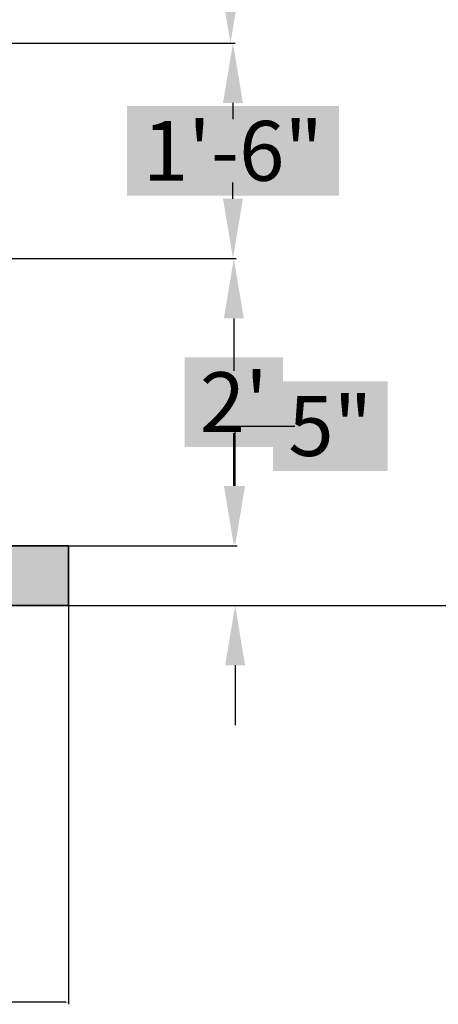
# Model space of a CAD drawing. Units: inches. Extents: x -301 to 715, y -607 to 364.
# Tile 32 of 141: x 159 to 194, y -574 to -492. Entities that reach past the tile are written whole.
import ezdxf

# ---------------------------------------------------------------- set-up
doc = ezdxf.new("R2010")
doc.units = ezdxf.units.IN
doc.header["$MEASUREMENT"] = 0
for name, color, linetype, lineweight in [('A-ANNO-DIMS', 2, 'Continuous', 18), ('A-SECT-PATT', 8, 'Continuous', 13), ('S-FNDN', 2, 'Continuous', 35)]:
    doc.layers.add(name, color=color, linetype=linetype, lineweight=lineweight)
doc.styles.get("Standard").update_dxf_attribs({"font": 'arial.ttf'})
doc.dimstyles.get("Standard").update_dxf_attribs({"dimtxt": 0.18, "dimasz": 0.18, "dimexe": 0.18, "dimexo": 0.0625, "dimgap": 0.09, "dimtad": 0, "dimtih": 1, "dimtoh": 1, "dimdec": 1, "dimzin": 0, "dimdsep": 46, "dimlunit": 4, "dimtxsty": 'Standard', "dimcen": 0.09, "dimclrd": 3, "dimclre": 4, "dimclrt": 6, "dimadec": 0, "dimazin": 0, "dimtfac": 1, "dimtdec": 1, "dimtofl": 0, "dimtmove": 0, "dimatfit": 3, "dimfxl": 1, "dimtfill": 2, "dimtfillclr": 51, "dimtolj": 1, "dimtzin": 0, "dimarcsym": 0})

# ---------------------------------------------------------------- blocks, each defined once
blk = doc.blocks.new('*D77')
at = {"layer": 'A-ANNO-DIMS', "color": 0, "lineweight": -2, "transparency": 16777216}
for p, q in [((177.201, -530.477), (177.201, -525.477)), ((177.201, -525.477), (182.201, -525.477)), ((163.318, -535.477), (177.381, -535.477)), ((163.318, -540.477), (177.381, -540.477)), ((177.201, -545.477), (177.201, -550.477))]:
    blk.add_line(p, q, dxfattribs=at)
at = {"layer": 'A-ANNO-DIMS', "color": 0, "transparency": 16777216}
for points in [[(176.368, -530.477), (178.035, -530.477), (177.201, -535.477)], [(176.368, -545.477), (178.035, -545.477), (177.201, -540.477)]]:
    blk.add_solid(points, dxfattribs=at)
at = {"layer": 'Defpoints', "color": 0, "transparency": 16777216}
for p in [(163.255, -535.477), (177.201, -535.477), (163.255, -540.477)]:
    blk.add_point(p, dxfattribs=at)
at = {"layer": 'A-ANNO-DIMS', "color": 0, "transparency": 16777216, "insert": (185.165, -525.477), "char_height": 5, "attachment_point": 5, "bg_fill": 1, "box_fill_scale": 1.25, "bg_fill_color": 51, "bg_fill_transparency": 0}
blk.add_mtext('\\A1;5"', dxfattribs=at)
blk = doc.blocks.new('*D78')
at = {"layer": 'A-ANNO-DIMS', "color": 0, "lineweight": -2, "transparency": 16777216}
for p, q in [((158.318, -511.477), (177.276, -511.477)), ((177.096, -516.477), (177.096, -520.877)), ((177.096, -530.477), (177.096, -526.078)), ((158.318, -535.477), (177.276, -535.477))]:
    blk.add_line(p, q, dxfattribs=at)
at = {"layer": 'A-ANNO-DIMS', "color": 0, "transparency": 16777216}
for points in [[(176.262, -516.477), (177.929, -516.477), (177.096, -511.477)], [(176.262, -530.477), (177.929, -530.477), (177.096, -535.477)]]:
    blk.add_solid(points, dxfattribs=at)
at = {"layer": 'Defpoints', "color": 0, "transparency": 16777216}
for p in [(158.255, -511.477), (177.096, -511.477), (158.255, -535.477)]:
    blk.add_point(p, dxfattribs=at)
at = {"layer": 'A-ANNO-DIMS', "color": 0, "transparency": 16777216, "insert": (177.096, -523.477), "char_height": 5, "attachment_point": 5, "bg_fill": 1, "box_fill_scale": 1.25, "bg_fill_color": 51, "bg_fill_transparency": 0}
blk.add_mtext("\\A1;2'", dxfattribs=at)
blk = doc.blocks.new('*D79')
at = {"layer": 'A-ANNO-DIMS', "color": 0, "lineweight": -2, "transparency": 16777216}
for p, q in [((153.318, -493.477), (177.201, -493.477)), ((177.021, -498.477), (177.021, -499.835)), ((177.021, -506.477), (177.021, -505.12)), ((153.318, -511.477), (177.201, -511.477))]:
    blk.add_line(p, q, dxfattribs=at)
at = {"layer": 'A-ANNO-DIMS', "color": 0, "transparency": 16777216}
for points in [[(176.188, -498.477), (177.854, -498.477), (177.021, -493.477)], [(176.188, -506.477), (177.854, -506.477), (177.021, -511.477)]]:
    blk.add_solid(points, dxfattribs=at)
at = {"layer": 'Defpoints', "color": 0, "transparency": 16777216}
for p in [(153.255, -493.477), (177.021, -493.477), (153.255, -511.477)]:
    blk.add_point(p, dxfattribs=at)
at = {"layer": 'A-ANNO-DIMS', "color": 0, "transparency": 16777216, "insert": (177.021, -502.477), "char_height": 5, "attachment_point": 5, "bg_fill": 1, "box_fill_scale": 1.25, "bg_fill_color": 51, "bg_fill_transparency": 0}
blk.add_mtext('\\A1;1\'-6"', dxfattribs=at)
blk = doc.blocks.new('*D80')
at = {"layer": 'A-ANNO-DIMS', "color": 0, "lineweight": -2, "transparency": 16777216}
for p, q in [((176.814, -481.477), (176.814, -476.477)), ((176.814, -476.477), (181.814, -476.477)), ((153.318, -481.477), (176.994, -481.477)), ((176.814, -488.477), (176.814, -486.477)), ((153.318, -493.477), (176.994, -493.477))]:
    blk.add_line(p, q, dxfattribs=at)
at = {"layer": 'A-ANNO-DIMS', "color": 0, "transparency": 16777216}
for points in [[(175.981, -486.477), (177.648, -486.477), (176.814, -481.477)], [(175.981, -488.477), (177.648, -488.477), (176.814, -493.477)]]:
    blk.add_solid(points, dxfattribs=at)
at = {"layer": 'Defpoints', "color": 0, "transparency": 16777216}
for p in [(153.255, -481.477), (176.814, -481.477), (153.255, -493.477)]:
    blk.add_point(p, dxfattribs=at)
at = {"layer": 'A-ANNO-DIMS', "color": 0, "transparency": 16777216, "insert": (183.969, -476.477), "char_height": 5, "attachment_point": 5, "bg_fill": 1, "box_fill_scale": 1.25, "bg_fill_color": 51, "bg_fill_transparency": 0}
blk.add_mtext("\\A1;1'", dxfattribs=at)
blk = doc.blocks.new('*D176')
at = {"layer": 'A-ANNO-DIMS', "color": 4, "lineweight": -2, "transparency": 16777216}
for p, q in [((148.28, -324.477), (215.605, -324.477)), ((-15.22, -540.477), (215.605, -540.477))]:
    blk.add_line(p, q, dxfattribs=at)
at = {"layer": 'A-ANNO-DIMS', "color": 3, "lineweight": -2, "transparency": 16777216}
for p, q in [((215.425, -324.657), (215.425, -432.296)), ((215.425, -540.297), (215.425, -432.659))]:
    blk.add_line(p, q, dxfattribs=at)
at = {"layer": 'A-ANNO-DIMS', "color": 3, "transparency": 16777216}
for points in [[(215.395, -324.657), (215.455, -324.657), (215.425, -324.477)], [(215.395, -540.297), (215.455, -540.297), (215.425, -540.477)]]:
    blk.add_solid(points, dxfattribs=at)
at = {"layer": 'Defpoints', "color": 0, "transparency": 16777216}
for p in [(148.218, -324.477), (-15.282, -540.477), (215.425, -540.477)]:
    blk.add_point(p, dxfattribs=at)
at = {"layer": 'A-ANNO-DIMS', "color": 6, "transparency": 16777216, "insert": (215.425, -432.477), "char_height": 0.18, "attachment_point": 5, "bg_fill": 1, "box_fill_scale": 1.25, "bg_fill_color": 51, "bg_fill_transparency": 0}
blk.add_mtext('\\A1;18\'-0"', dxfattribs=at)
blk = doc.blocks.new('*D182')
at = {"layer": 'A-ANNO-DIMS', "color": 4, "lineweight": -2, "transparency": 16777216}
for p, q in [((114.255, -540.54), (114.255, -573.809)), ((163.255, -540.54), (163.255, -573.809))]:
    blk.add_line(p, q, dxfattribs=at)
at = {"layer": 'A-ANNO-DIMS', "color": 3, "lineweight": -2, "transparency": 16777216}
for p, q in [((114.435, -573.629), (138.422, -573.629)), ((163.075, -573.629), (139.088, -573.629))]:
    blk.add_line(p, q, dxfattribs=at)
at = {"layer": 'A-ANNO-DIMS', "color": 3, "transparency": 16777216}
for points in [[(114.435, -573.599), (114.435, -573.659), (114.255, -573.629)], [(163.075, -573.599), (163.075, -573.659), (163.255, -573.629)]]:
    blk.add_solid(points, dxfattribs=at)
at = {"layer": 'Defpoints', "color": 0, "transparency": 16777216}
for p in [(114.255, -540.477), (163.255, -540.477), (163.255, -573.629)]:
    blk.add_point(p, dxfattribs=at)
at = {"layer": 'A-ANNO-DIMS', "color": 6, "transparency": 16777216, "insert": (138.755, -573.629), "char_height": 0.18, "attachment_point": 5, "bg_fill": 1, "box_fill_scale": 1.25, "bg_fill_color": 51, "bg_fill_transparency": 0}
blk.add_mtext('\\A1;4\'-1"', dxfattribs=at)

msp = doc.modelspace()

# ---------------------------------------------------------------- hatches: boundary and pattern name
at = {"layer": 'A-SECT-PATT'}
h = msp.add_hatch(dxfattribs=at)
h.set_pattern_fill('AR-CONC', color=256, scale=0.5)
h.set_pattern_definition([(50, (10.3213, 33.8764), (3.586301, -0.31376), [0.375, -4.125]), (355, (10.3213, 33.8764), (-0.693757, 3.76096), [0.3, -3.3]), (100.45144, (10.62, 33.8502), (2.892544, 3.4472), [0.3187, -3.50571]), (46.1842, (10.3213, 34.8764), (5.336207, -0.827596), [0.5625, -6.1875]), (96.6356, (10.766, 34.8074), (4.67331, 4.870593), [0.47805, -5.25857]), (351.1842, (10.321, 34.8764), (4.67331, 4.870593), [0.45, -4.95]), (21, (10.8213, 34.6264), (2.984535, -2.013094), [0.375, -4.125]), (326, (10.8213, 34.6264), (1.216577, 3.62575), [0.3, -3.3]), (71.45144, (11.07, 34.4586), (4.201112, 1.612656), [0.3187, -3.50571]), (37.5, (10.3213, 33.8764), (0.0607993, 1.6644693), [0, -3.26, 0, -3.35, 0, -3.3125]), (7.5, (10.3213, 33.8764), (1.3153477, 1.9720586), [0, -1.91, 0, -3.185, 0, -1.2625]), (327.5, (9.2063, 33.8764), (2.6691122, -0.1127744), [0, -1.25, 0, -3.9, 0, -5.175]), (317.5, (8.7063, 33.8764), (2.915931, 0.500525), [0, -1.625, 0, -2.59, 0, -3.675])])
h.paths.add_polyline_path([(-56.282, -535.477), (-61.282, -535.477), (-61.282, -540.477), (-15.282, -540.477), (-15.282, -535.477), (-20.282, -535.477)])
h.paths.add_polyline_path([(119.255, -535.477), (114.255, -535.477), (114.255, -540.477), (163.255, -540.477), (163.255, -535.477), (158.255, -535.477)])
h.paths.add_polyline_path([(-206.282, -471.477), (-209.282, -471.477), (-209.282, -481.477), (-206.282, -481.477), (-194.282, -481.477), (-194.282, -471.477)])
h.paths.add_polyline_path([(-41.282, -481.477), (-41.282, -471.477), (-185.282, -471.477), (-185.282, -481.477), (-180.282, -481.477)])
h.paths.add_polyline_path([(134.255, -481.477), (134.255, -471.477), (-35.282, -471.477), (-35.282, -481.477), (-30.282, -481.477)])
h.paths.add_polyline_path([(155.218, -481.477), (158.218, -481.477), (158.218, -471.477), (153.218, -471.477), (143.218, -471.477), (143.218, -481.477), (148.255, -481.477)])
h.paths.add_polyline_path([(-193.88, -356.477), (-193.904, -361.477), (143.218, -361.477), (143.218, -356.477)])

# ---------------------------------------------------------------- linework, layer by layer
at = {"layer": 'S-FNDN'}
for p, q in [((158.255, -535.477), (163.255, -535.477)), ((163.255, -535.477), (163.255, -540.477)), ((114.255, -540.477), (163.255, -540.477))]:
    msp.add_line(p, q, dxfattribs=at)

# ---------------------------------------------------------------- dimensions: what is measured, and where the dimension line sits
at = {"layer": 'A-ANNO-DIMS'}
for base, p1, p2, override, picture, middle in [((215.425, -540.477), (148.218, -324.477), (-15.282, -540.477), {"dimdec": 1, "dimlfac": 1, "dimrnd": 0, "dimzin": 1, "dimdsep": 46, "dimlunit": 4, "dimfrac": 2}, '*D176', (215.425, -432.477)), ((176.814, -481.477), (153.255, -493.477), (153.255, -481.477), {"dimtxt": 5, "dimasz": 5, "dimclrd": 0, "dimclre": 0, "dimclrt": 0}, '*D80', (183.969, -476.477)), ((177.021, -493.477), (153.255, -511.477), (153.255, -493.477), {"dimtxt": 5, "dimasz": 5, "dimclrd": 0, "dimclre": 0, "dimclrt": 0}, '*D79', (177.021, -502.477)), ((177.096, -511.477), (158.255, -535.477), (158.255, -511.477), {"dimtxt": 5, "dimasz": 5, "dimclrd": 0, "dimclre": 0, "dimclrt": 0}, '*D78', (177.096, -523.477)), ((177.201, -535.477), (163.255, -540.477), (163.255, -535.477), {"dimtxt": 5, "dimasz": 5, "dimclrd": 0, "dimclre": 0, "dimclrt": 0}, '*D77', (185.165, -525.477))]:
    dim = msp.add_linear_dim(base=base, p1=p1, p2=p2, angle=90, dimstyle='Standard', override=override, dxfattribs=at)
    dim.commit()
    dim.dimension.update_dxf_attribs({"geometry": picture, "text_midpoint": middle})
dim = msp.add_linear_dim(base=(163.255, -573.629), p1=(114.255, -540.477), p2=(163.255, -540.477), dimstyle='Standard', override={"dimdec": 1, "dimlfac": 1, "dimrnd": 0, "dimzin": 1, "dimdsep": 46, "dimlunit": 4, "dimfrac": 2}, dxfattribs=at)
dim.commit()
dim.dimension.update_dxf_attribs({"geometry": '*D182', "text_midpoint": (138.755, -573.629)})

doc.saveas('drawing.dxf')
